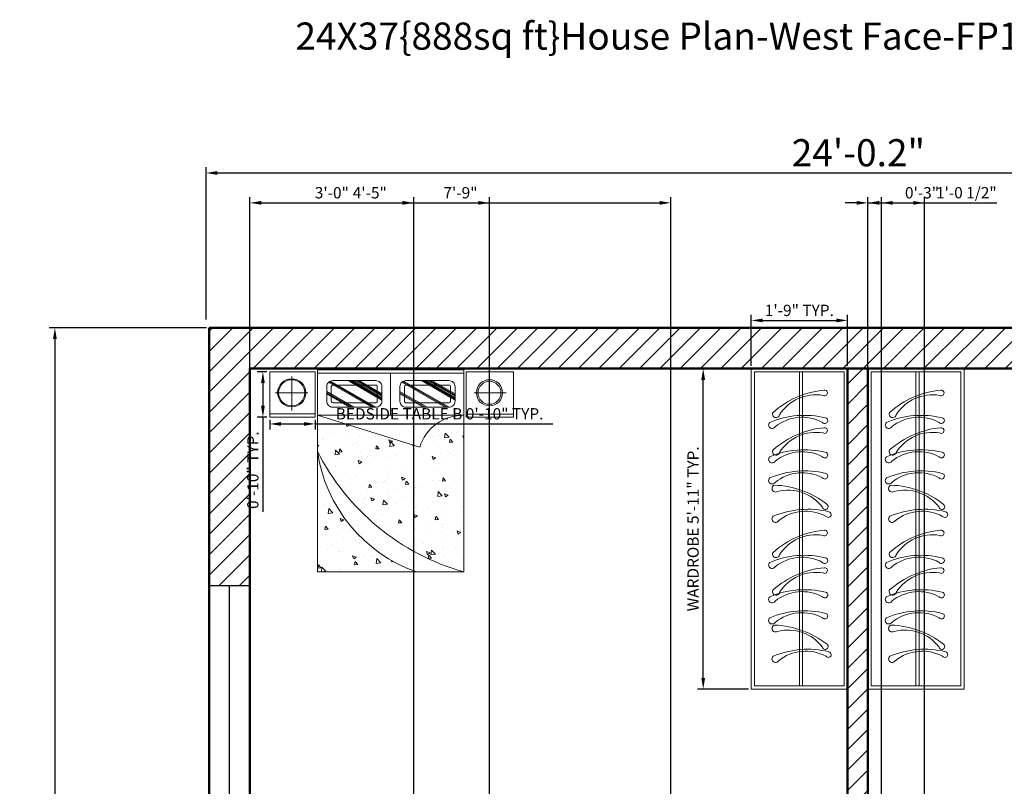
# Model space of a CAD drawing. Units: inches. Extents: x 3064 to 3516, y 2736 to 3280.
# Tile 4 of 5: x 3106 to 3324, y 3110 to 3280. Entities that reach past the tile are written whole.
import ezdxf

# ---------------------------------------------------------------- set-up
doc = ezdxf.new("R2010")
doc.units = ezdxf.units.IN
for name, color, linetype, lineweight in [('A-ANNO-DIMS', 2, 'Continuous', 18), ('A-ANNO-TEXT', 7, 'Continuous', 25), ('A-FURN', 8, 'Continuous', 18), ('A-FURN-PATT', 9, 'Continuous', 13), ('A-GLAZ', 5, 'Continuous', 25), ('A-WALL', 7, 'Continuous', 50), ('A-WALL-PATT', 8, 'Continuous', 13)]:
    doc.layers.add(name, color=color, linetype=linetype, lineweight=lineweight)
doc.styles.get("Standard").update_dxf_attribs({"font": 'arial.ttf'})
doc.dimstyles.new('ISO-25', dxfattribs={"dimtxt": 2.5, "dimasz": 2.5, "dimexe": 1.25, "dimexo": 0.625, "dimtad": 1, "dimlunit": 3, "dimtxsty": 'Standard', "dimcen": 2.5, "dimadec": 0, "dimazin": 0, "dimtfac": 1, "dimtmove": 0, "dimatfit": 3, "dimfxl": 1, "dimarcsym": 0})

# ---------------------------------------------------------------- blocks, each defined once
blk = doc.blocks.new('*D3')
at = {"layer": 'A-ANNO-DIMS', "color": 0, "lineweight": -2, "transparency": 16777216}
for p, q in [((3147.2, 3213.35), (3147.2, 3246.96)), ((3149.7, 3245.71), (3432.9, 3245.71)), ((3435.4, 3212.14), (3435.4, 3246.96))]:
    blk.add_line(p, q, dxfattribs=at)
at = {"layer": 'A-ANNO-DIMS', "color": 0, "transparency": 16777216}
for points in [[(3149.7, 3246.13), (3149.7, 3245.3), (3147.2, 3245.71)], [(3432.9, 3246.13), (3432.9, 3245.3), (3435.4, 3245.71)]]:
    blk.add_solid(points, dxfattribs=at)
at = {"layer": 'Defpoints', "color": 0, "transparency": 16777216}
for p in [(3435.4, 3245.71), (3147.2, 3212.72), (3435.4, 3211.51)]:
    blk.add_point(p, dxfattribs=at)
at = {"layer": 'A-ANNO-DIMS', "color": 0, "transparency": 16777216, "insert": (3291.3, 3249.4), "char_height": 6, "attachment_point": 5}
blk.add_mtext('24\'-0.2"', dxfattribs=at)
blk = doc.blocks.new('*D4')
at = {"layer": 'A-ANNO-DIMS', "color": 0, "lineweight": -2, "transparency": 16777216}
for p, q in [((3147.27, 3211.51), (3112.57, 3211.51)), ((3113.82, 3209.01), (3113.82, 2771.51)), ((3147.27, 2769.01), (3112.57, 2769.01))]:
    blk.add_line(p, q, dxfattribs=at)
at = {"layer": 'A-ANNO-DIMS', "color": 0, "transparency": 16777216}
for points in [[(3113.4, 3209.01), (3114.23, 3209.01), (3113.82, 3211.51)], [(3113.4, 2771.51), (3114.23, 2771.51), (3113.82, 2769.01)]]:
    blk.add_solid(points, dxfattribs=at)
at = {"layer": 'Defpoints', "color": 0, "transparency": 16777216}
for p in [(3147.9, 3211.51), (3113.82, 2769.01), (3147.9, 2769.01)]:
    blk.add_point(p, dxfattribs=at)
at = {"layer": 'A-ANNO-DIMS', "color": 0, "transparency": 16777216, "insert": (3110.13, 2990.26), "char_height": 6, "attachment_point": 5, "rotation": 90}
blk.add_mtext('36\'-10.5"', dxfattribs=at)
blk = doc.blocks.new('WIN-60IN')
for p, q in [((0, 60), (0, 0)), ((9, 60), (0, 60)), ((4.5, 60), (4.5, 0)), ((9, 0), (9, 60)), ((0, 0), (9, 0))]:
    blk.add_line(p, q)
blk = doc.blocks.new('BEDSIDE-TABLE-A')
for p, q in [((0, 0), (0, 10.49)), ((0, 10.49), (10.04, 10.49)), ((4.67, 1.81), (4.67, 8.9)), ((9.38, 0), (9.38, 10.49)), ((10.04, 10.49), (10.04, 0)), ((1.1, 5.18), (8.23, 5.18)), ((10.04, 0), (0, 0))]:
    blk.add_line(p, q)
for radius in [2.89, 2.54]:
    blk.add_circle((4.67, 5.18), radius)
blk = doc.blocks.new('BEDSIDE-TABLE-B')
for p, q in [((10.04, 10.04), (0, 10.04)), ((0, 10.04), (0, 0)), ((9.34, 0), (9.34, 10.04)), ((10.04, 0), (10.04, 10.04)), ((4.67, 1.21), (4.67, 8.43)), ((1.04, 4.86), (8.55, 4.86)), ((0, 0), (10.04, 0))]:
    blk.add_line(p, q)
for radius in [3.11, 2.89]:
    blk.add_circle((4.67, 4.86), radius)
blk = doc.blocks.new('WARDROBE-HANGING')
for p, q in [((0, 0), (0, 70.83)), ((0, 70.83), (21.25, 70.83)), ((0.71, 0.71), (0.71, 70.12)), ((0.71, 70.12), (20.54, 70.12)), ((10.62, 70.12), (10.62, 0.71)), ((11.33, 70.12), (11.33, 0.71)), ((20.54, 70.12), (20.54, 0.71)), ((21.25, 70.83), (21.25, 0)), ((10.62, 0.71), (0.71, 0.71)), ((20.54, 0.71), (10.62, 0.71)), ((21.25, 0), (0, 0))]:
    blk.add_line(p, q)
for points in [[(16.12, 66.06, -1.400346), (15.85, 64.9, 0.30346), (6.22, 60.57, -1.157387), (4.8, 61.14, -0.160871)], [(16.4, 59.93, -1.400346), (15.76, 58.92, 0.30346), (5.25, 57.94, -1.157387), (4.09, 58.94, -0.160871)], [(16.12, 57.76, -1.400346), (15.85, 56.6, 0.30346), (6.22, 52.27, -1.157387), (4.8, 52.84, -0.160871)], [(16.4, 52.33, -1.400346), (15.76, 51.32, 0.30346), (5.25, 50.34, -1.157387), (4.09, 51.34, -0.160871)], [(16.4, 47.67, -1.400346), (15.76, 46.66, 0.30346), (5.25, 45.68, -1.157387), (4.09, 46.67, -0.160871)], [(16.73, 40.83, -1.400346), (15.72, 40.18, 0.30346), (5.77, 43.67, -1.157387), (5.13, 45.07, -0.160871)], [(17.15, 39.19, -1.400346), (16.51, 38.18, 0.30346), (6.01, 37.19, -1.157387), (4.84, 38.19, -0.160871)], [(16.12, 35.14, -1.400346), (15.85, 33.98, 0.30346), (6.22, 29.65, -1.157387), (4.8, 30.22, -0.160871)], [(16.4, 29.01, -1.400346), (15.76, 28, 0.30346), (5.25, 27.02, -1.157387), (4.09, 28.02, -0.160871)], [(16.12, 26.84, -1.400346), (15.85, 25.68, 0.30346), (6.22, 21.35, -1.157387), (4.8, 21.92, -0.160871)], [(16.4, 21.42, -1.400346), (15.76, 20.4, 0.30346), (5.25, 19.42, -1.157387), (4.09, 20.42, -0.160871)], [(16.4, 16.75, -1.400346), (15.76, 15.74, 0.30346), (5.25, 14.76, -1.157387), (4.09, 15.76, -0.160871)], [(16.73, 9.91, -1.400346), (15.72, 9.26, 0.30346), (5.77, 12.76, -1.157387), (5.13, 14.15, -0.160871)], [(17.15, 8.27, -1.400346), (16.51, 7.26, 0.30346), (6.01, 6.27, -1.157387), (4.84, 7.27, -0.160871)]]:
    blk.add_lwpolyline(points, format="xyb", close=True)
blk = doc.blocks.new('BED-FRAME-AND-COVER')
for p, q in [((0, 32.36), (44.63, 32.36)), ((0, 0), (0, 32.36)), ((0.73, 0), (0.73, 32.36)), ((10.02, 0), (10.02, 32.36)), ((44.63, 32.36), (44.63, 0)), ((10.02, 0), (17.09, 22.61)), ((10.02, 16.18), (0.73, 16.18)), ((44.63, 0), (0, 0))]:
    blk.add_line(p, q)
for centre, radius, start, end in [((20, 32.16), 9.98, 178.8468, 253.0453), ((-5.57, 46.57), 52.17, 296.7955, 344.1914), ((13.16, 33.03), 33.38, 278.2583, 340.5572)]:
    blk.add_arc(centre, radius, start, end)
blk = doc.blocks.new('*D27')
at = {"layer": 'A-ANNO-DIMS', "color": 0, "lineweight": -2, "transparency": 16777216}
for p, q in [((3161.27, 3191.16), (3161.27, 3189.03)), ((3171.31, 3191.16), (3171.31, 3189.03)), ((3163.77, 3190.28), (3168.81, 3190.28)), ((3171.31, 3190.28), (3223.77, 3190.28))]:
    blk.add_line(p, q, dxfattribs=at)
at = {"layer": 'A-ANNO-DIMS', "color": 0, "transparency": 16777216}
for points in [[(3163.77, 3190.69), (3163.77, 3189.86), (3161.27, 3190.28)], [(3168.81, 3190.69), (3168.81, 3189.86), (3171.31, 3190.28)]]:
    blk.add_solid(points, dxfattribs=at)
at = {"layer": 'Defpoints', "color": 0, "transparency": 16777216}
for p in [(3161.27, 3191.78), (3171.31, 3191.78), (3171.31, 3190.28)]:
    blk.add_point(p, dxfattribs=at)
at = {"layer": 'A-ANNO-DIMS', "color": 0, "transparency": 16777216, "insert": (3198.79, 3192.19), "char_height": 2.5, "attachment_point": 5}
blk.add_mtext('BEDSIDE TABLE B 0\'-10" TYP.', dxfattribs=at)
blk = doc.blocks.new('*D28')
at = {"layer": 'A-ANNO-DIMS', "color": 0, "lineweight": -2, "transparency": 16777216}
for p, q in [((3160.64, 3201.82), (3158.51, 3201.82)), ((3159.76, 3199.32), (3159.76, 3194.28)), ((3160.64, 3191.78), (3158.51, 3191.78)), ((3159.76, 3191.78), (3159.76, 3170.85))]:
    blk.add_line(p, q, dxfattribs=at)
at = {"layer": 'A-ANNO-DIMS', "color": 0, "transparency": 16777216}
for points in [[(3159.35, 3199.32), (3160.18, 3199.32), (3159.76, 3201.82)], [(3159.35, 3194.28), (3160.18, 3194.28), (3159.76, 3191.78)]]:
    blk.add_solid(points, dxfattribs=at)
at = {"layer": 'Defpoints', "color": 0, "transparency": 16777216}
for p in [(3161.27, 3201.82), (3159.76, 3191.78), (3161.27, 3191.78)]:
    blk.add_point(p, dxfattribs=at)
at = {"layer": 'A-ANNO-DIMS', "color": 0, "transparency": 16777216, "insert": (3157.86, 3180.07), "char_height": 2.5, "attachment_point": 5, "rotation": 90}
blk.add_mtext('0\'-10" TYP.', dxfattribs=at)
blk = doc.blocks.new('*D31')
at = {"layer": 'A-ANNO-DIMS', "color": 0, "lineweight": -2, "transparency": 16777216}
for p, q in [((3267.02, 3202.51), (3255.77, 3202.51)), ((3257.02, 3134.19), (3257.02, 3200.01)), ((3267.02, 3131.69), (3255.77, 3131.69))]:
    blk.add_line(p, q, dxfattribs=at)
at = {"layer": 'A-ANNO-DIMS', "color": 0, "transparency": 16777216}
for points in [[(3256.6, 3200.01), (3257.43, 3200.01), (3257.02, 3202.51)], [(3256.6, 3134.19), (3257.43, 3134.19), (3257.02, 3131.69)]]:
    blk.add_solid(points, dxfattribs=at)
at = {"layer": 'Defpoints', "color": 0, "transparency": 16777216}
for p in [(3257.02, 3202.51), (3267.64, 3202.51), (3267.64, 3131.69)]:
    blk.add_point(p, dxfattribs=at)
at = {"layer": 'A-ANNO-DIMS', "color": 0, "transparency": 16777216, "insert": (3255.1, 3167.1), "char_height": 2.5, "attachment_point": 5, "rotation": 90}
blk.add_mtext('WARDROBE 5\'-11" TYP.', dxfattribs=at)
blk = doc.blocks.new('*D32')
at = {"layer": 'A-ANNO-DIMS', "color": 0, "lineweight": -2, "transparency": 16777216}
for p, q in [((3267.64, 3203.14), (3267.64, 3214.39)), ((3270.14, 3213.14), (3286.39, 3213.14)), ((3288.89, 3203.14), (3288.89, 3214.39))]:
    blk.add_line(p, q, dxfattribs=at)
at = {"layer": 'A-ANNO-DIMS', "color": 0, "transparency": 16777216}
for points in [[(3270.14, 3213.56), (3270.14, 3212.72), (3267.64, 3213.14)], [(3286.39, 3213.56), (3286.39, 3212.72), (3288.89, 3213.14)]]:
    blk.add_solid(points, dxfattribs=at)
at = {"layer": 'Defpoints', "color": 0, "transparency": 16777216}
for p in [(3288.89, 3213.14), (3267.64, 3202.51), (3288.89, 3202.51)]:
    blk.add_point(p, dxfattribs=at)
at = {"layer": 'A-ANNO-DIMS', "color": 0, "transparency": 16777216, "insert": (3278.26, 3215.04), "char_height": 2.5, "attachment_point": 5}
blk.add_mtext('1\'-9" TYP.', dxfattribs=at)
blk = doc.blocks.new('*D50')
at = {"layer": 'A-ANNO-DIMS', "color": 0, "lineweight": -2, "transparency": 16777216}
for p, q in [((3156.9, 3030.78), (3156.9, 3240.36)), ((3159.4, 3239.11), (3190.59, 3239.11)), ((3193.09, 3030.78), (3193.09, 3240.36))]:
    blk.add_line(p, q, dxfattribs=at)
at = {"layer": 'A-ANNO-DIMS', "color": 0, "transparency": 16777216}
for points in [[(3159.4, 3239.53), (3159.4, 3238.7), (3156.9, 3239.11)], [(3190.59, 3239.53), (3190.59, 3238.7), (3193.09, 3239.11)]]:
    blk.add_solid(points, dxfattribs=at)
at = {"layer": 'Defpoints', "color": 0, "transparency": 16777216}
for p in [(3193.09, 3239.11), (3156.9, 3030.16), (3193.09, 3030.16)]:
    blk.add_point(p, dxfattribs=at)
at = {"layer": 'A-ANNO-DIMS', "color": 0, "transparency": 16777216, "insert": (3174.99, 3241.02), "char_height": 2.5, "attachment_point": 5}
blk.add_mtext('3\'-0"', dxfattribs=at)
blk = doc.blocks.new('*D52')
at = {"layer": 'A-ANNO-DIMS', "color": 0, "lineweight": -2, "transparency": 16777216}
for p, q in [((3156.9, 2964.64), (3156.9, 3240.36)), ((3159.4, 3239.11), (3207.34, 3239.11)), ((3209.84, 2964.64), (3209.84, 3240.36))]:
    blk.add_line(p, q, dxfattribs=at)
at = {"layer": 'A-ANNO-DIMS', "color": 0, "transparency": 16777216}
for points in [[(3159.4, 3239.53), (3159.4, 3238.7), (3156.9, 3239.11)], [(3207.34, 3239.53), (3207.34, 3238.7), (3209.84, 3239.11)]]:
    blk.add_solid(points, dxfattribs=at)
at = {"layer": 'Defpoints', "color": 0, "transparency": 16777216}
for p in [(3209.84, 3239.11), (3156.9, 2964.01), (3209.84, 2964.01)]:
    blk.add_point(p, dxfattribs=at)
at = {"layer": 'A-ANNO-DIMS', "color": 0, "transparency": 16777216, "insert": (3183.37, 3241.01), "char_height": 2.5, "attachment_point": 5}
blk.add_mtext('4\'-5"', dxfattribs=at)
blk = doc.blocks.new('*D57')
at = {"layer": 'A-ANNO-DIMS', "color": 0, "lineweight": -2, "transparency": 16777216}
for p, q in [((3156.9, 3047.14), (3156.9, 3240.36)), ((3159.4, 3239.11), (3247.4, 3239.11)), ((3249.9, 3047.14), (3249.9, 3240.36))]:
    blk.add_line(p, q, dxfattribs=at)
at = {"layer": 'A-ANNO-DIMS', "color": 0, "transparency": 16777216}
for points in [[(3159.4, 3239.53), (3159.4, 3238.7), (3156.9, 3239.11)], [(3247.4, 3239.53), (3247.4, 3238.7), (3249.9, 3239.11)]]:
    blk.add_solid(points, dxfattribs=at)
at = {"layer": 'Defpoints', "color": 0, "transparency": 16777216}
for p in [(3249.9, 3239.11), (3156.9, 3046.51), (3249.9, 3046.51)]:
    blk.add_point(p, dxfattribs=at)
at = {"layer": 'A-ANNO-DIMS', "color": 0, "transparency": 16777216, "insert": (3203.4, 3241.02), "char_height": 2.5, "attachment_point": 5}
blk.add_mtext('7\'-9"', dxfattribs=at)
blk = doc.blocks.new('*D61')
at = {"layer": 'A-ANNO-DIMS', "color": 0, "lineweight": -2, "transparency": 16777216}
for p, q in [((3293.4, 2861.14), (3293.4, 3240.36)), ((3295.9, 3239.11), (3303.4, 3239.11)), ((3305.9, 2861.14), (3305.9, 3240.36)), ((3305.9, 3239.11), (3321.88, 3239.11))]:
    blk.add_line(p, q, dxfattribs=at)
at = {"layer": 'A-ANNO-DIMS', "color": 0, "transparency": 16777216}
for points in [[(3295.9, 3239.53), (3295.9, 3238.7), (3293.4, 3239.11)], [(3303.4, 3239.53), (3303.4, 3238.7), (3305.9, 3239.11)]]:
    blk.add_solid(points, dxfattribs=at)
at = {"layer": 'Defpoints', "color": 0, "transparency": 16777216}
for p in [(3305.9, 3239.11), (3293.4, 2860.51), (3305.9, 2860.51)]:
    blk.add_point(p, dxfattribs=at)
at = {"layer": 'A-ANNO-DIMS', "color": 0, "transparency": 16777216, "insert": (3315.14, 3241.03), "char_height": 2.5, "attachment_point": 5}
blk.add_mtext('1\'-0 1/2"', dxfattribs=at)
blk = doc.blocks.new('*D62')
at = {"layer": 'A-ANNO-DIMS', "color": 0, "lineweight": -2, "transparency": 16777216}
for p, q in [((3290.9, 3239.11), (3288.4, 3239.11)), ((3293.4, 3047.14), (3293.4, 3240.36)), ((3293.4, 3239.11), (3296.4, 3239.11)), ((3296.4, 3047.14), (3296.4, 3240.36)), ((3298.9, 3239.11), (3309.29, 3239.11))]:
    blk.add_line(p, q, dxfattribs=at)
at = {"layer": 'A-ANNO-DIMS', "color": 0, "transparency": 16777216}
for points in [[(3290.9, 3239.53), (3290.9, 3238.7), (3293.4, 3239.11)], [(3298.9, 3239.53), (3298.9, 3238.7), (3296.4, 3239.11)]]:
    blk.add_solid(points, dxfattribs=at)
at = {"layer": 'Defpoints', "color": 0, "transparency": 16777216}
for p in [(3296.4, 3239.11), (3293.4, 3046.51), (3296.4, 3046.51)]:
    blk.add_point(p, dxfattribs=at)
at = {"layer": 'A-ANNO-DIMS', "color": 0, "transparency": 16777216, "insert": (3305.35, 3241.02), "char_height": 2.5, "attachment_point": 5}
blk.add_mtext('0\'-3"', dxfattribs=at)

msp = doc.modelspace()

# ---------------------------------------------------------------- hatches: boundary and pattern name
at = {"layer": 'A-FURN-PATT'}
h = msp.add_hatch(dxfattribs=at)
h.set_pattern_fill('ANSI31', color=256, scale=0.0702853387, angle=105.041628, style=0)
h.paths.add_polyline_path([(3184.783, 3193.971), (3184.702, 3193.971), (3184.256, 3193.971), (3183.809, 3193.971), (3183.728, 3193.971), (3174.219, 3199.451), (3174.253, 3199.479), (3174.438, 3199.629), (3174.669, 3199.754), (3174.71, 3199.776)])
h = msp.add_hatch(dxfattribs=at)
h.set_pattern_fill('ANSI31', color=256, scale=0.0702858852, angle=105.041628, style=0)
h.paths.add_polyline_path([(3186.027, 3196.126), (3186.027, 3196.08), (3186.027, 3195.822), (3186.027, 3195.564), (3186.027, 3195.518), (3178.497, 3199.858), (3178.578, 3199.858), (3179.024, 3199.858), (3179.471, 3199.858), (3179.552, 3199.858)])
h = msp.add_hatch(dxfattribs=at)
h.set_pattern_fill('ANSI31', color=256, scale=0.0702831553, angle=105.041628, style=0)
h.paths.add_polyline_path([(3186.027, 3196.961), (3186.027, 3196.914), (3186.027, 3196.657), (3186.027, 3196.399), (3186.027, 3196.353), (3179.946, 3199.858), (3180.026, 3199.858), (3180.473, 3199.858), (3180.92, 3199.858), (3181, 3199.858)])
h = msp.add_hatch(dxfattribs=at)
h.set_pattern_fill('ANSI31', color=256, scale=0.0702860721, angle=105.041628, style=0)
h.paths.add_polyline_path([(3200.962, 3193.971), (3200.881, 3193.971), (3200.434, 3193.971), (3199.988, 3193.971), (3199.907, 3193.971), (3190.398, 3199.451), (3190.431, 3199.479), (3190.617, 3199.629), (3190.847, 3199.754), (3190.889, 3199.776)])
h = msp.add_hatch(dxfattribs=at)
h.set_pattern_fill('ANSI31', color=256, scale=0.0702830263, angle=105.041628, style=0)
h.paths.add_polyline_path([(3202.206, 3196.126), (3202.206, 3196.08), (3202.206, 3195.822), (3202.206, 3195.564), (3202.206, 3195.518), (3194.676, 3199.858), (3194.756, 3199.858), (3195.203, 3199.858), (3195.65, 3199.858), (3195.73, 3199.858)])
h = msp.add_hatch(dxfattribs=at)
h.set_pattern_fill('ANSI31', color=256, scale=0.0702838921, angle=105.041628, style=0)
h.paths.add_polyline_path([(3202.206, 3196.961), (3202.206, 3196.914), (3202.206, 3196.657), (3202.206, 3196.399), (3202.206, 3196.353), (3196.124, 3199.858), (3196.205, 3199.858), (3196.651, 3199.858), (3197.098, 3199.858), (3197.179, 3199.858)])
h = msp.add_hatch(dxfattribs=at)
h.set_pattern_fill('ANSI31', color=256, scale=0.0702858391, angle=105.041628, style=0)
h.paths.add_polyline_path([(3179.929, 3193.971), (3179.849, 3193.971), (3179.402, 3193.971), (3178.955, 3193.971), (3178.875, 3193.971), (3173.848, 3196.868), (3173.848, 3196.914), (3173.848, 3197.172), (3173.848, 3197.43), (3173.848, 3197.476)])
h = msp.add_hatch(dxfattribs=at)
h.set_pattern_fill('ANSI31', color=256, scale=0.0702865719, angle=105.041628, style=0)
h.paths.add_polyline_path([(3196.108, 3193.971), (3196.028, 3193.971), (3195.581, 3193.971), (3195.134, 3193.971), (3195.054, 3193.971), (3190.027, 3196.868), (3190.027, 3196.914), (3190.027, 3197.172), (3190.027, 3197.43), (3190.027, 3197.476)])
h = msp.add_hatch(dxfattribs=at)
h.set_pattern_fill('AR-CONC', color=256, scale=0.044631, angle=360, style=0)
h.set_pattern_definition([(130, (3585.4047, 669.415), (-8.131058, -0.711375), [0.850218, -9.352396]), (185, (3585.405, 669.415), (1.572917, 8.527021), [0.680174, -7.481917]), (79.549, (3584.727, 669.356), (-6.55817, 7.815608), [0.722574, -7.94831]), (133.8158, (3585.405, 671.682), (-12.09849, -1.876385), [1.275327, -14.028594]), (83.3644, (3584.396, 671.526), (-10.595554, 11.042814), [1.08386, -11.922464]), (188.816, (3585.405, 671.682), (-10.59557, 11.042795), [1.02026, -11.222875]), (159, (3584.271, 671.1155), (-6.766702, -4.564198), [0.850218, -9.352396]), (214, (3584.271, 671.1155), (-2.758277, 8.220467), [0.680174, -7.481917]), (108.5486, (3583.707, 670.735), (-9.52496, 3.656287), [0.722574, -7.94831]), (142.5, (3585.4047, 669.415), (-0.137847, 3.7737637), [0, -7.391227, 0, -7.595279, 0, -7.510257]), (172.5, (3585.4047, 669.415), (-2.982219, 4.471145), [0, -4.330443, 0, -7.221183, 0, -2.8624]), (212.5, (3587.9326, 669.415), (-6.0515243, -0.2556787), [0, -2.834059, 0, -8.842265, 0, -11.733006]), (222.5, (3589.0663, 669.415), (-6.611132, 1.134806), [0, -3.684277, 0, -5.872171, 0, -8.332134])])
edge = h.paths.add_edge_path()
edge.add_ellipse((3203.949, 3182.214), major_axis=(7.055, -7.055), ratio=1, start_angle=136.15316, end_angle=208.04534, ccw=False)
edge.add_line((3203.748, 3192.19), (3204.15, 3192.19))
edge.add_line((3204.15, 3192.19), (3204.15, 3157.579))
edge.add_ellipse((3218.363, 3207.779), major_axis=(36.892, -36.892), ratio=1, start_angle=251.7955, end_angle=299.1914, ccw=False)
edge.add_line((3171.792, 3184.259), (3171.792, 3192.19))
edge.add_line((3171.792, 3192.19), (3194.405, 3185.124))
edge = h.paths.add_edge_path()
edge.add_line((3193.713, 3157.579), (3171.792, 3157.579))
edge.add_line((3171.792, 3157.579), (3171.792, 3184.259))
edge.add_ellipse((3204.823, 3189.053), major_axis=(-23.601, -23.601), ratio=1, start_angle=323.25827, end_angle=385.55722)
at = {"layer": 'A-WALL-PATT'}
h = msp.add_hatch(dxfattribs=at)
h.set_pattern_fill('ANSI31', color=256)
h.paths.add_polyline_path([(3156.897, 2985.015), (3147.897, 2985.015), (3147.897, 2923.515), (3156.897, 2923.515)])
h.paths.add_polyline_path([(3156.897, 2863.515), (3147.897, 2863.515), (3147.897, 2812.515), (3156.897, 2812.515)])
h.paths.add_polyline_path([(3293.397, 2778.015), (3239.397, 2778.015), (3239.397, 2780.015), (3234.897, 2780.015), (3234.897, 2778.015), (3156.897, 2778.015), (3156.897, 2788.515), (3147.897, 2788.515), (3147.897, 2769.015), (3293.397, 2769.015)])
h.paths.add_polyline_path([(3369.397, 2778.015), (3343.897, 2778.015), (3344.15, 2769.015), (3369.397, 2769.015)])
h.paths.add_polyline_path([(3435.397, 2788.515), (3426.397, 2788.515), (3426.397, 2778.015), (3405.397, 2778.015), (3405.397, 2769.015), (3435.397, 2769.015)])
h.paths.add_polyline_path([(3435.397, 2960.265), (3426.397, 2960.265), (3426.397, 2812.515), (3435.397, 2812.515)])
h.paths.add_polyline_path([(3435.397, 3094.515), (3426.397, 3094.515), (3426.397, 3020.265), (3435.397, 3020.265)])
h.paths.add_polyline_path([(3435.397, 3211.515), (3147.897, 3211.515), (3147.897, 3154.515), (3156.897, 3154.515), (3156.897, 3202.515), (3426.397, 3202.515), (3426.397, 3154.515), (3435.397, 3154.515)])
h.paths.add_polyline_path([(3293.397, 3202.515), (3288.897, 3202.515), (3288.897, 3046.515), (3285.897, 3046.515), (3285.897, 3042.015), (3296.397, 3042.015), (3296.397, 3046.515), (3293.397, 3046.515)])
h.paths.add_polyline_path([(3426.397, 3046.515), (3332.397, 3046.515), (3332.397, 3042.015), (3426.397, 3042.015)])
h.paths.add_polyline_path([(3249.897, 3046.515), (3156.897, 3046.515), (3156.897, 3042.015), (3249.897, 3042.015)])
h.paths.add_polyline_path([(3156.897, 3094.515), (3147.897, 3094.515), (3147.897, 3021.015), (3156.897, 3021.015)])
h.paths.add_polyline_path([(3293.397, 2964.015), (3156.897, 2964.015), (3156.897, 2959.515), (3288.897, 2959.515), (3288.897, 2956.515), (3293.397, 2956.515)])
h.paths.add_polyline_path([(3249.897, 2827.515), (3156.897, 2827.515), (3156.897, 2823.015), (3234.897, 2823.015), (3234.897, 2816.015), (3239.397, 2816.015), (3239.397, 2823.015), (3249.897, 2823.015)])
h.paths.add_polyline_path([(3293.397, 2920.515), (3288.897, 2920.515), (3288.897, 2827.515), (3285.897, 2827.515), (3285.897, 2823.015), (3293.397, 2823.015), (3293.397, 2856.015), (3305.897, 2856.015), (3305.897, 2860.515), (3293.397, 2860.515)])
h.paths.add_polyline_path([(3348.397, 2920.515), (3343.897, 2920.515), (3343.897, 2860.515), (3341.897, 2860.515), (3341.897, 2856.015), (3343.897, 2856.015), (3343.897, 2778.015), (3348.397, 2778.015), (3348.397, 2823.015), (3350.397, 2823.015), (3350.397, 2827.515), (3348.397, 2827.515)])
h.paths.add_polyline_path([(3426.397, 2827.515), (3386.397, 2827.515), (3386.397, 2823.015), (3426.397, 2823.015)])

# ---------------------------------------------------------------- linework, layer by layer
at = {"layer": 'A-FURN'}
for points in [[(3184.688, 3199.858), (3175.187, 3199.858, 0.4142136), (3173.848, 3198.519), (3173.848, 3195.309, 0.4142136), (3175.187, 3193.971), (3184.688, 3193.971, 0.4142136), (3186.027, 3195.309), (3186.027, 3198.519, 0.4142136)], [(3200.867, 3199.858), (3191.366, 3199.858, 0.4142136), (3190.027, 3198.519), (3190.027, 3195.309, 0.4142136), (3191.366, 3193.971), (3200.867, 3193.971, 0.4142136), (3202.206, 3195.309), (3202.206, 3198.519, 0.4142136)], [(3184.688, 3198.854), (3175.187, 3198.854, 0.4142136), (3174.852, 3198.519), (3174.852, 3195.309, 0.4142136), (3175.187, 3194.975), (3184.688, 3194.975, 0.4142136), (3185.023, 3195.309), (3185.023, 3198.519, 0.4142136)], [(3200.867, 3198.854), (3191.366, 3198.854, 0.4142136), (3191.031, 3198.519), (3191.031, 3195.309, 0.4142136), (3191.366, 3194.975), (3200.867, 3194.975, 0.4142136), (3201.202, 3195.309), (3201.202, 3198.519, 0.4142136)]]:
    msp.add_lwpolyline(points, format="xyb", close=True, dxfattribs=at)
at = {"layer": 'A-WALL'}
for p, q in [((3147.897, 3211.515), (3147.897, 2769.015)), ((3147.897, 3211.515), (3435.397, 3211.515)), ((3156.897, 3202.515), (3426.397, 3202.515)), ((3156.897, 3202.515), (3156.897, 2778.015)), ((3288.897, 3202.515), (3288.897, 3046.515)), ((3293.397, 3202.515), (3293.397, 3046.515))]:
    msp.add_line(p, q, dxfattribs=at)

# ---------------------------------------------------------------- block references
at = {"layer": 'A-FURN'}
for name, p, rotation in [('BEDSIDE-TABLE-B', (3161.269, 3201.823), 269.9999999999973), ('BED-FRAME-AND-COVER', (3171.792, 3202.21), 269.9999999999995), ('BEDSIDE-TABLE-A', (3204.631, 3201.823), 270)]:
    msp.add_blockref(name, p, dxfattribs=dict(at, rotation=rotation))
for p in [(3267.64, 3131.687), (3293.4, 3131.687)]:
    msp.add_blockref('WARDROBE-HANGING', p, dxfattribs=at)
at = {"layer": 'A-GLAZ', "rotation": 180}
msp.add_blockref('WIN-60IN', (3156.897, 3154.515), dxfattribs=at)

# ---------------------------------------------------------------- texts
at = {"layer": 'A-ANNO-TEXT', "insert": (3166.949, 3278.95), "char_height": 6, "attachment_point": 1}
msp.add_mtext_dynamic_manual_height_columns('24X37\\{888sq ft\\}House Plan-West Face-FP1323', width=332.43103, gutter_width=12.5, heights=[0], dxfattribs=at)

# ---------------------------------------------------------------- dimensions: what is measured, and where the dimension line sits
at = {"layer": 'A-ANNO-DIMS'}
for base, p1, p2, override, picture, middle in [((3435.397, 3245.713), (3147.2, 3212.723), (3435.397, 3211.515), {"dimtxt": 6, "dimclrd": 0, "dimclre": 0, "dimclrt": 0}, '*D3', (3291.299, 3249.402)), ((3305.897, 3239.115), (3293.397, 2860.515), (3305.897, 2860.515), {"dimdec": 1, "dimlfac": 1, "dimrnd": 0, "dimzin": 1, "dimdsep": 46, "dimlunit": 4, "dimfrac": 2}, '*D61', (3315.14, 3241.033)), ((3193.09, 3239.115), (3156.897, 3030.159), (3193.09, 3030.159), {"dimdec": 1, "dimlfac": 1, "dimrnd": 0, "dimzin": 1, "dimdsep": 46, "dimlunit": 4, "dimfrac": 2}, '*D50', (3174.994, 3241.017)), ((3249.897, 3239.115), (3156.897, 3046.515), (3249.897, 3046.515), {"dimdec": 1, "dimlfac": 1, "dimrnd": 0, "dimzin": 1, "dimdsep": 46, "dimlunit": 4, "dimfrac": 2}, '*D57', (3203.397, 3241.016)), ((3209.842, 3239.115), (3156.897, 2964.015), (3209.842, 2964.015), {"dimdec": 1, "dimlfac": 1, "dimrnd": 0, "dimzin": 1, "dimdsep": 46, "dimlunit": 4, "dimfrac": 2}, '*D52', (3183.37, 3241.011)), ((3296.397, 3239.115), (3293.397, 3046.515), (3296.397, 3046.515), {"dimdec": 1, "dimlfac": 1, "dimrnd": 0, "dimzin": 1, "dimdsep": 46, "dimlunit": 4, "dimfrac": 2}, '*D62', (3305.345, 3241.017))]:
    dim = msp.add_linear_dim(base=base, p1=p1, p2=p2, dimstyle='ISO-25', override=override, dxfattribs=at)
    dim.commit()
    dim.dimension.update_dxf_attribs({"geometry": picture, "text_midpoint": middle})
for base, p1, p2, text, picture, middle in [((3288.889, 3213.139), (3267.64, 3202.515), (3288.889, 3202.515), '<> TYP.', '*D32', (3278.265, 3215.041)), ((3171.311, 3190.275), (3161.269, 3191.781), (3171.311, 3191.781), 'BEDSIDE TABLE B <> TYP.', '*D27', (3198.79, 3192.193))]:
    dim = msp.add_linear_dim(base=base, p1=p1, p2=p2, text=text, dimstyle='ISO-25', override={"dimdec": 1, "dimlfac": 1, "dimrnd": 0, "dimzin": 1, "dimdsep": 46, "dimlunit": 4, "dimfrac": 2}, dxfattribs=at)
    dim.commit()
    dim.dimension.update_dxf_attribs({"geometry": picture, "text_midpoint": middle})
dim = msp.add_linear_dim(base=(3113.817, 2769.015), p1=(3147.897, 3211.515), p2=(3147.897, 2769.015), angle=90, dimstyle='ISO-25', override={"dimtxt": 6, "dimclrd": 0, "dimclre": 0, "dimclrt": 0}, dxfattribs=at)
dim.commit()
dim.dimension.update_dxf_attribs({"geometry": '*D4', "text_midpoint": (3110.126, 2990.265)})
for base, p1, p2, angle, text, picture, middle in [((3159.763, 3191.781), (3161.269, 3201.823), (3161.269, 3191.781), 270, '<> TYP.', '*D28', (3157.861, 3180.066)), ((3257.016, 3202.515), (3267.64, 3131.687), (3267.64, 3202.515), 90, 'WARDROBE <> TYP.', '*D31', (3255.098, 3167.101))]:
    dim = msp.add_linear_dim(base=base, p1=p1, p2=p2, angle=angle, text=text, dimstyle='ISO-25', override={"dimdec": 1, "dimlfac": 1, "dimrnd": 0, "dimzin": 1, "dimdsep": 46, "dimlunit": 4, "dimfrac": 2}, dxfattribs=at)
    dim.commit()
    dim.dimension.update_dxf_attribs({"geometry": picture, "text_midpoint": middle})

doc.saveas('drawing.dxf')
